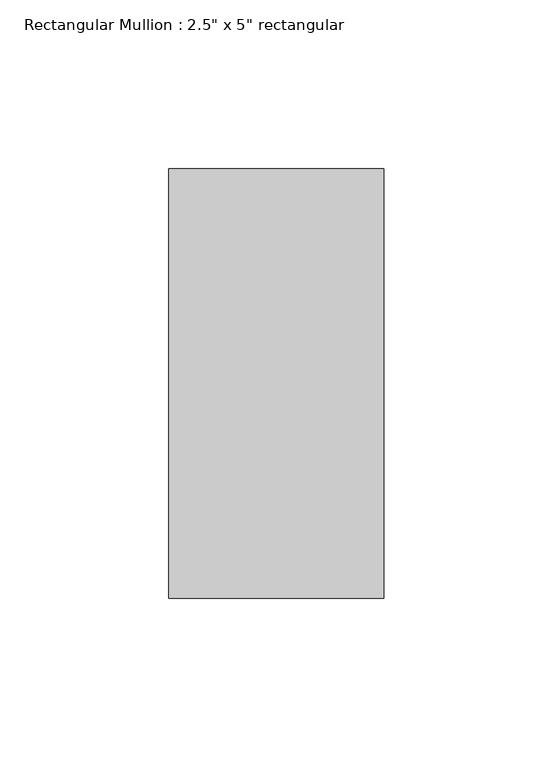
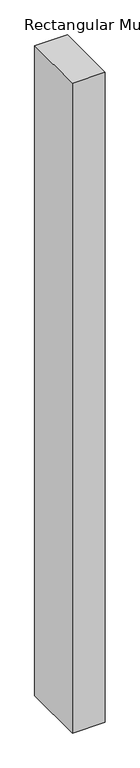
"""IFC4 building model written with IfcOpenShell, lengths in millimetres: member geometry."""

from ifc_helpers import new_model, si_unit, frame, origin, place, context, project, spatial, polyline, outline, extrude, source, transform, mapped, element, save


def member_709922c8(model_context):
    return source(origin(), model_context, "Body", "SweptSolid", [
        extrude(outline(polyline([(31.75, 63.5), (31.75, -63.5), (-31.75, -63.5), (-31.75, 63.5), (31.75, 63.5)])), frame((0.0, 0.0, -1334.3185135), z_axis=(0.0, 0.0, 1.0), x_axis=(1.0, 0.0, 0.0)), (0.0, 0.0, 1.0), 1334.3185135),
    ])


if __name__ == "__main__":
    model = new_model("IFC4")
    model_context = context("Model", 3, world=origin())
    ifc_project = project(units=[si_unit("LENGTHUNIT", "METRE", prefix="MILLI")], contexts=[model_context])
    site = spatial("IfcSite", under=ifc_project)
    building = spatial("IfcBuilding", under=site)
    placement = place(None, origin())
    member_shape = member_709922c8(model_context)
    element("IfcMember", 1, ObjectType="Rectangular Mullion : 2.5\" x 5\" rectangular", at=placement, inside=building, context=model_context, shape_type="MappedRepresentation", body=[
        mapped(member_shape, transform((0.0, 0.0, 0.0), x_axis=(1.0, 0.0, 0.0), y_axis=(0.0, 1.0, 0.0), z_axis=(0.0, 0.0, 1.0))),
    ])
    save(model, "model.ifc")

# Revit data of these elements
# Type "Rectangular Mullion : 2.5\" x 5\" rectangular"
#   built-in parameter 1007304 = 0.416667 (stored number, unit not read)
#   built-in parameter 1007301 = 0.104167 (stored number, unit not read)
#   built-in parameter 1007300 = 0.104167 (stored number, unit not read)
# Element 1 (IfcMember, "Rectangular Mullion : 2.5\" x 5\" rectangular")
#   Materials on its faces: "Aluminum"
# Materials
#   "Aluminum": class "Metal", colour RGB 247 247 247, transparency 0, Description = "Aluminum 6061", Cost = 0
